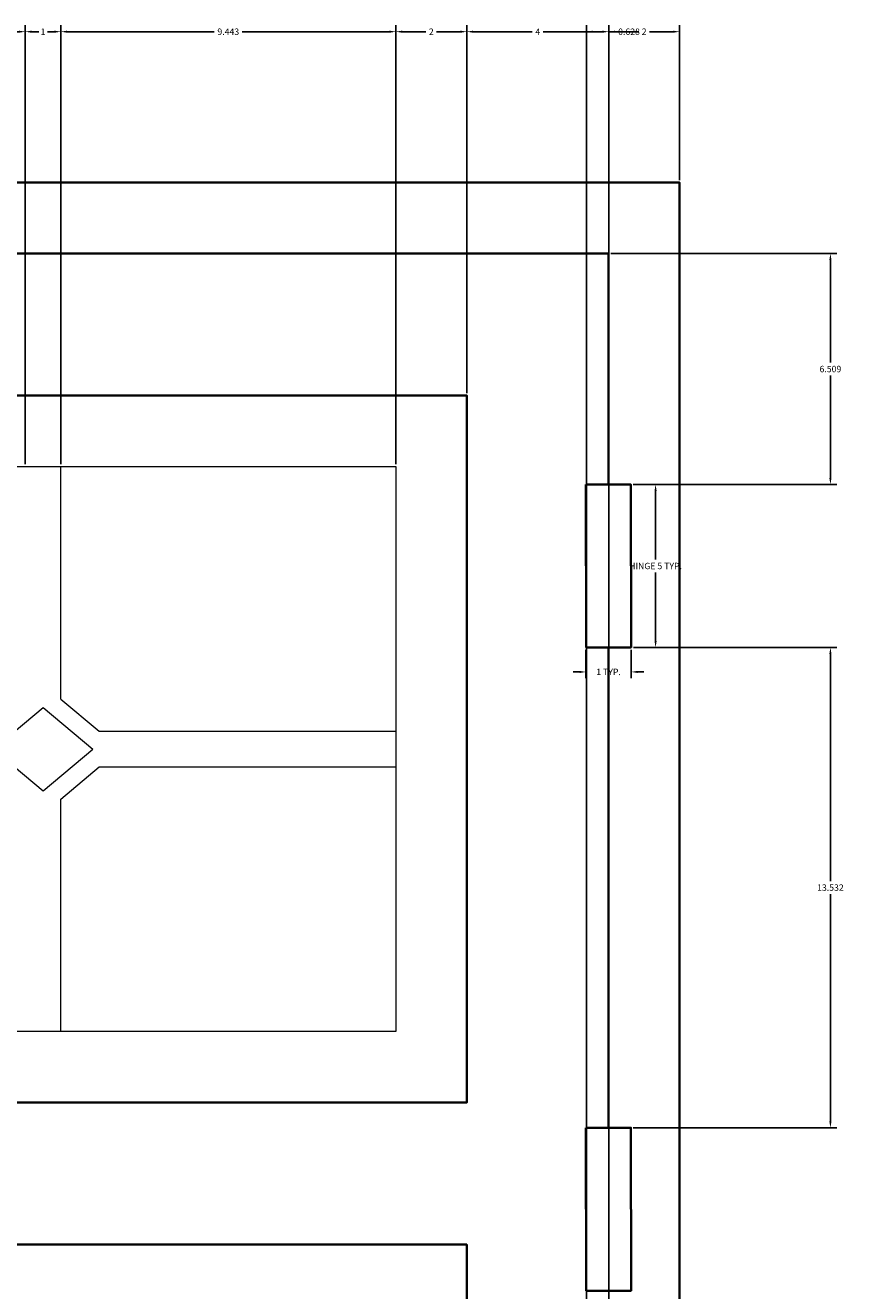
# Model space of a CAD drawing. Units: inches. Extents: x 3137 to 3299, y 1994 to 2089.
# Tile 7 of 14: x 3171 to 3194, y 2052 to 2087. Entities that reach past the tile are written whole.
import ezdxf

# ---------------------------------------------------------------- set-up
doc = ezdxf.new("R2010")
doc.units = ezdxf.units.IN
doc.header["$MEASUREMENT"] = 0
for name, color, linetype, lineweight in [('A-ANNO-DIMS', 2, 'Continuous', 18), ('A-DOOR', 4, 'Continuous', 35), ('A-GLAZ', 3, 'Continuous', 18)]:
    doc.layers.add(name, color=color, linetype=linetype, lineweight=lineweight)
doc.styles.get("Standard").update_dxf_attribs({"font": 'arial.ttf'})
doc.dimstyles.get("Standard").update_dxf_attribs({"dimtxt": 0.18, "dimasz": 0.18, "dimexe": 0.18, "dimexo": 0.0625, "dimgap": 0.09, "dimtad": 0, "dimtih": 1, "dimtoh": 1, "dimdec": 4, "dimzin": 0, "dimdsep": 46, "dimtxsty": 'Standard', "dimcen": 0.09, "dimadec": 0, "dimazin": 0, "dimtfac": 1, "dimtdec": 4, "dimtofl": 0, "dimtmove": 0, "dimatfit": 3, "dimfxl": 1, "dimtolj": 1, "dimtzin": 0, "dimarcsym": 0})

# ---------------------------------------------------------------- blocks, each defined once
blk = doc.blocks.new('GLAZ-DIAMOND-MOTIF')
for points in [[(0, 1.174), (1.407, 2.349)], [(1.407, 2.349), (2.809, 1.174)], [(0, 1.174), (1.407, 0)], [(1.407, 0), (2.809, 1.174)]]:
    blk.add_lwpolyline(points)
blk = doc.blocks.new('DOOR-HINGE')
blk.add_lwpolyline([(0, 4.592), (1.268, 4.592), (1.275, 0), (0.007, 0)], close=True)
blk = doc.blocks.new('*D5')
at = {"layer": 'A-ANNO-DIMS', "color": 0, "lineweight": -2, "transparency": 16777216}
for p, q in [((3188.174, 2074.365), (3188.98, 2074.365)), ((3188.8, 2074.185), (3188.8, 2072.252)), ((3188.8, 2069.953), (3188.8, 2071.886)), ((3188.174, 2069.773), (3188.98, 2069.773))]:
    blk.add_line(p, q, dxfattribs=at)
at = {"layer": 'A-ANNO-DIMS', "color": 0, "transparency": 16777216}
for points in [[(3188.77, 2074.185), (3188.83, 2074.185), (3188.8, 2074.365)], [(3188.77, 2069.953), (3188.83, 2069.953), (3188.8, 2069.773)]]:
    blk.add_solid(points, dxfattribs=at)
at = {"layer": 'Defpoints', "color": 0, "transparency": 16777216}
for p in [(3188.112, 2074.365), (3188.8, 2074.365), (3188.112, 2069.773)]:
    blk.add_point(p, dxfattribs=at)
at = {"layer": 'A-ANNO-DIMS', "color": 0, "transparency": 16777216, "insert": (3188.8, 2072.069), "char_height": 0.18, "attachment_point": 5}
blk.add_mtext('\\A1;HINGE 5 TYP.', dxfattribs=at)
blk = doc.blocks.new('*D6')
at = {"layer": 'A-ANNO-DIMS', "color": 0, "lineweight": -2, "transparency": 16777216}
for p, q in [((3186.837, 2069.711), (3186.837, 2068.904)), ((3188.112, 2069.711), (3188.112, 2068.904)), ((3186.657, 2069.084), (3186.477, 2069.084)), ((3188.292, 2069.084), (3188.472, 2069.084))]:
    blk.add_line(p, q, dxfattribs=at)
at = {"layer": 'A-ANNO-DIMS', "color": 0, "transparency": 16777216}
for points in [[(3186.657, 2069.114), (3186.657, 2069.054), (3186.837, 2069.084)], [(3188.292, 2069.114), (3188.292, 2069.054), (3188.112, 2069.084)]]:
    blk.add_solid(points, dxfattribs=at)
at = {"layer": 'Defpoints', "color": 0, "transparency": 16777216}
for p in [(3186.837, 2069.773), (3188.112, 2069.773), (3188.112, 2069.084)]:
    blk.add_point(p, dxfattribs=at)
at = {"layer": 'A-ANNO-DIMS', "color": 0, "transparency": 16777216, "insert": (3187.475, 2069.084), "char_height": 0.18, "attachment_point": 5}
blk.add_mtext('\\A1;1 TYP.', dxfattribs=at)
blk = doc.blocks.new('*D28')
at = {"layer": 'A-ANNO-DIMS', "color": 0, "lineweight": -2, "transparency": 16777216}
for p, q in [((3159.858, 2074.936), (3159.858, 2087.304)), ((3171.035, 2074.936), (3171.035, 2087.304)), ((3160.038, 2087.124), (3164.991, 2087.124)), ((3170.855, 2087.124), (3165.902, 2087.124))]:
    blk.add_line(p, q, dxfattribs=at)
at = {"layer": 'A-ANNO-DIMS', "color": 0, "transparency": 16777216}
for points in [[(3160.038, 2087.154), (3160.038, 2087.094), (3159.858, 2087.124)], [(3170.855, 2087.154), (3170.855, 2087.094), (3171.035, 2087.124)]]:
    blk.add_solid(points, dxfattribs=at)
at = {"layer": 'Defpoints', "color": 0, "transparency": 16777216}
for p in [(3171.035, 2087.124), (3159.858, 2074.874), (3171.035, 2074.874)]:
    blk.add_point(p, dxfattribs=at)
at = {"layer": 'A-ANNO-DIMS', "color": 0, "transparency": 16777216, "insert": (3165.446, 2087.124), "char_height": 0.18, "attachment_point": 5}
blk.add_mtext('\\A1;11.177', dxfattribs=at)
blk = doc.blocks.new('*D29')
at = {"layer": 'A-ANNO-DIMS', "color": 0, "lineweight": -2, "transparency": 16777216}
for p, q in [((3171.035, 2074.936), (3171.035, 2087.304)), ((3172.035, 2074.936), (3172.035, 2087.304)), ((3171.215, 2087.124), (3171.412, 2087.124)), ((3171.855, 2087.124), (3171.658, 2087.124))]:
    blk.add_line(p, q, dxfattribs=at)
at = {"layer": 'A-ANNO-DIMS', "color": 0, "transparency": 16777216}
for points in [[(3171.215, 2087.154), (3171.215, 2087.094), (3171.035, 2087.124)], [(3171.855, 2087.154), (3171.855, 2087.094), (3172.035, 2087.124)]]:
    blk.add_solid(points, dxfattribs=at)
at = {"layer": 'Defpoints', "color": 0, "transparency": 16777216}
for p in [(3172.035, 2087.124), (3171.035, 2074.874), (3172.035, 2074.874)]:
    blk.add_point(p, dxfattribs=at)
at = {"layer": 'A-ANNO-DIMS', "color": 0, "transparency": 16777216, "insert": (3171.535, 2087.124), "char_height": 0.18, "attachment_point": 5}
blk.add_mtext('\\A1;1', dxfattribs=at)
blk = doc.blocks.new('*D30')
at = {"layer": 'A-ANNO-DIMS', "color": 0, "lineweight": -2, "transparency": 16777216}
for p, q in [((3172.035, 2074.936), (3172.035, 2087.304)), ((3181.478, 2074.936), (3181.478, 2087.304)), ((3172.215, 2087.124), (3176.363, 2087.124)), ((3181.298, 2087.124), (3177.15, 2087.124))]:
    blk.add_line(p, q, dxfattribs=at)
at = {"layer": 'A-ANNO-DIMS', "color": 0, "transparency": 16777216}
for points in [[(3172.215, 2087.154), (3172.215, 2087.094), (3172.035, 2087.124)], [(3181.298, 2087.154), (3181.298, 2087.094), (3181.478, 2087.124)]]:
    blk.add_solid(points, dxfattribs=at)
at = {"layer": 'Defpoints', "color": 0, "transparency": 16777216}
for p in [(3181.478, 2087.124), (3172.035, 2074.874), (3181.478, 2074.874)]:
    blk.add_point(p, dxfattribs=at)
at = {"layer": 'A-ANNO-DIMS', "color": 0, "transparency": 16777216, "insert": (3176.756, 2087.124), "char_height": 0.18, "attachment_point": 5}
blk.add_mtext('\\A1;9.443', dxfattribs=at)
blk = doc.blocks.new('*D31')
at = {"layer": 'A-ANNO-DIMS', "color": 0, "lineweight": -2, "transparency": 16777216}
for p, q in [((3181.478, 2074.936), (3181.478, 2087.304)), ((3183.478, 2076.936), (3183.478, 2087.304)), ((3181.658, 2087.124), (3182.328, 2087.124)), ((3183.298, 2087.124), (3182.627, 2087.124))]:
    blk.add_line(p, q, dxfattribs=at)
at = {"layer": 'A-ANNO-DIMS', "color": 0, "transparency": 16777216}
for points in [[(3181.658, 2087.154), (3181.658, 2087.094), (3181.478, 2087.124)], [(3183.298, 2087.154), (3183.298, 2087.094), (3183.478, 2087.124)]]:
    blk.add_solid(points, dxfattribs=at)
at = {"layer": 'Defpoints', "color": 0, "transparency": 16777216}
for p in [(3183.478, 2087.124), (3183.478, 2076.874), (3181.478, 2074.874)]:
    blk.add_point(p, dxfattribs=at)
at = {"layer": 'A-ANNO-DIMS', "color": 0, "transparency": 16777216, "insert": (3182.478, 2087.124), "char_height": 0.18, "attachment_point": 5}
blk.add_mtext('\\A1;2', dxfattribs=at)
blk = doc.blocks.new('*D32')
at = {"layer": 'A-ANNO-DIMS', "color": 0, "lineweight": -2, "transparency": 16777216}
for p, q in [((3183.478, 2076.936), (3183.478, 2087.304)), ((3187.478, 2080.936), (3187.478, 2087.304)), ((3183.658, 2087.124), (3185.325, 2087.124)), ((3187.298, 2087.124), (3185.63, 2087.124))]:
    blk.add_line(p, q, dxfattribs=at)
at = {"layer": 'A-ANNO-DIMS', "color": 0, "transparency": 16777216}
for points in [[(3183.658, 2087.154), (3183.658, 2087.094), (3183.478, 2087.124)], [(3187.298, 2087.154), (3187.298, 2087.094), (3187.478, 2087.124)]]:
    blk.add_solid(points, dxfattribs=at)
at = {"layer": 'Defpoints', "color": 0, "transparency": 16777216}
for p in [(3187.478, 2087.124), (3187.478, 2080.874), (3183.478, 2076.874)]:
    blk.add_point(p, dxfattribs=at)
at = {"layer": 'A-ANNO-DIMS', "color": 0, "transparency": 16777216, "insert": (3185.478, 2087.124), "char_height": 0.18, "attachment_point": 5}
blk.add_mtext('\\A1;4', dxfattribs=at)
blk = doc.blocks.new('*D33')
at = {"layer": 'A-ANNO-DIMS', "color": 0, "lineweight": -2, "transparency": 16777216}
for p, q in [((3187.478, 2080.936), (3187.478, 2087.304)), ((3189.478, 2082.936), (3189.478, 2087.304)), ((3187.658, 2087.124), (3188.328, 2087.124)), ((3189.298, 2087.124), (3188.627, 2087.124))]:
    blk.add_line(p, q, dxfattribs=at)
at = {"layer": 'A-ANNO-DIMS', "color": 0, "transparency": 16777216}
for points in [[(3187.658, 2087.154), (3187.658, 2087.094), (3187.478, 2087.124)], [(3189.298, 2087.154), (3189.298, 2087.094), (3189.478, 2087.124)]]:
    blk.add_solid(points, dxfattribs=at)
at = {"layer": 'Defpoints', "color": 0, "transparency": 16777216}
for p in [(3189.478, 2087.124), (3189.478, 2082.874), (3187.478, 2080.874)]:
    blk.add_point(p, dxfattribs=at)
at = {"layer": 'A-ANNO-DIMS', "color": 0, "transparency": 16777216, "insert": (3188.478, 2087.124), "char_height": 0.18, "attachment_point": 5}
blk.add_mtext('\\A1;2', dxfattribs=at)
blk = doc.blocks.new('*D53')
at = {"layer": 'A-ANNO-DIMS', "color": 0, "lineweight": -2, "transparency": 16777216}
for p, q in [((3188.174, 2069.773), (3193.908, 2069.773)), ((3193.728, 2069.593), (3193.728, 2063.189)), ((3193.728, 2056.421), (3193.728, 2062.825)), ((3188.168, 2056.241), (3193.908, 2056.241))]:
    blk.add_line(p, q, dxfattribs=at)
at = {"layer": 'A-ANNO-DIMS', "color": 0, "transparency": 16777216}
for points in [[(3193.698, 2069.593), (3193.758, 2069.593), (3193.728, 2069.773)], [(3193.698, 2056.421), (3193.758, 2056.421), (3193.728, 2056.241)]]:
    blk.add_solid(points, dxfattribs=at)
at = {"layer": 'Defpoints', "color": 0, "transparency": 16777216}
for p in [(3188.112, 2069.773), (3193.728, 2069.773), (3188.105, 2056.241)]:
    blk.add_point(p, dxfattribs=at)
at = {"layer": 'A-ANNO-DIMS', "color": 0, "transparency": 16777216, "insert": (3193.728, 2063.007), "char_height": 0.18, "attachment_point": 5}
blk.add_mtext('\\A1;13.532', dxfattribs=at)
blk = doc.blocks.new('*D54')
at = {"layer": 'A-ANNO-DIMS', "color": 0, "lineweight": -2, "transparency": 16777216}
for p, q in [((3187.54, 2080.874), (3193.908, 2080.874)), ((3193.728, 2080.694), (3193.728, 2077.801)), ((3193.728, 2074.545), (3193.728, 2077.438)), ((3188.168, 2074.365), (3193.908, 2074.365))]:
    blk.add_line(p, q, dxfattribs=at)
at = {"layer": 'A-ANNO-DIMS', "color": 0, "transparency": 16777216}
for points in [[(3193.698, 2080.694), (3193.758, 2080.694), (3193.728, 2080.874)], [(3193.698, 2074.545), (3193.758, 2074.545), (3193.728, 2074.365)]]:
    blk.add_solid(points, dxfattribs=at)
at = {"layer": 'Defpoints', "color": 0, "transparency": 16777216}
for p in [(3187.478, 2080.874), (3193.728, 2080.874), (3188.105, 2074.365)]:
    blk.add_point(p, dxfattribs=at)
at = {"layer": 'A-ANNO-DIMS', "color": 0, "transparency": 16777216, "insert": (3193.728, 2077.619), "char_height": 0.18, "attachment_point": 5}
blk.add_mtext('\\A1;6.509', dxfattribs=at)
blk = doc.blocks.new('*D76')
at = {"layer": 'A-ANNO-DIMS', "color": 0, "lineweight": -2, "transparency": 16777216}
for p, q in [((3186.849, 2012.332), (3186.849, 2087.304)), ((3187.478, 2012.332), (3187.478, 2087.304)), ((3187.029, 2087.124), (3187.298, 2087.124)), ((3187.478, 2087.124), (3187.658, 2087.124))]:
    blk.add_line(p, q, dxfattribs=at)
at = {"layer": 'A-ANNO-DIMS', "color": 0, "transparency": 16777216}
for points in [[(3187.029, 2087.154), (3187.029, 2087.094), (3186.849, 2087.124)], [(3187.298, 2087.154), (3187.298, 2087.094), (3187.478, 2087.124)]]:
    blk.add_solid(points, dxfattribs=at)
at = {"layer": 'Defpoints', "color": 0, "transparency": 16777216}
for p in [(3187.478, 2087.124), (3186.849, 2012.269), (3187.478, 2012.269)]:
    blk.add_point(p, dxfattribs=at)
at = {"layer": 'A-ANNO-DIMS', "color": 0, "transparency": 16777216, "insert": (3188.052, 2087.124), "char_height": 0.18, "attachment_point": 5}
blk.add_mtext('\\A1;0.628', dxfattribs=at)

msp = doc.modelspace()

# ---------------------------------------------------------------- linework, layer by layer
at = {"layer": 'A-DOOR'}
for points in [[(3141.4777, 2082.874), (3189.4777, 2082.874), (3189.4777, 1998.874), (3141.4777, 1998.874)], [(3147.4777, 2056.9483), (3147.4777, 2076.874), (3183.4777, 2076.874), (3183.4777, 2056.9483)], [(3147.4777, 2032.1375), (3147.4777, 2052.9483), (3183.4777, 2052.9483), (3183.4777, 2032.1375)]]:
    msp.add_lwpolyline(points, close=True, dxfattribs=at)
for points in [[(3187.4777, 2007.6773), (3187.4777, 2000.874), (3143.4777, 2000.874), (3143.4777, 2080.874), (3187.4777, 2080.874), (3187.4777, 2076.298)], [(3187.4777, 2080.874), (3187.4777, 2074.365)], [(3187.4777, 2069.7731), (3187.4777, 2056.2413)], [(3187.3375, 2056.2413), (3187.6053, 2056.2413)]]:
    msp.add_lwpolyline(points, dxfattribs=at)
at = {"layer": 'A-GLAZ'}
for p, q in [((3172.0351, 2068.3193), (3172.0351, 2074.874)), ((3173.1196, 2067.4111), (3181.4777, 2067.4111)), ((3173.1196, 2066.4111), (3181.4777, 2066.4111)), ((3172.0351, 2058.9483), (3172.0351, 2065.5029))]:
    msp.add_line(p, q, dxfattribs=at)
msp.add_lwpolyline([(3149.4777, 2058.9483), (3149.4777, 2074.874), (3181.4777, 2074.874), (3181.4777, 2058.9483)], close=True, dxfattribs=at)
for points in [[(3172.0351, 2068.3193), (3173.1196, 2067.4111)], [(3172.0351, 2065.5029), (3173.1196, 2066.4111)]]:
    msp.add_lwpolyline(points, dxfattribs=at)

# ---------------------------------------------------------------- block references
at = {"layer": 'A-DOOR'}
for p in [(3186.837, 2069.773), (3186.837, 2051.6493)]:
    msp.add_blockref('DOOR-HINGE', p, dxfattribs=at)
at = {"layer": 'A-GLAZ'}
msp.add_blockref('GLAZ-DIAMOND-MOTIF', (3170.1284, 2065.737), dxfattribs=at)

# ---------------------------------------------------------------- dimensions: what is measured, and where the dimension line sits
at = {"layer": 'A-ANNO-DIMS'}
for base, p1, p2, override, picture, middle in [((3171.0351, 2087.124), (3159.8577, 2074.874), (3171.0351, 2074.874), {"dimdec": 3, "dimlfac": 1, "dimrnd": 0, "dimzin": 0, "dimdsep": 46, "dimlunit": 2}, '*D28', (3165.4464, 2087.124)), ((3172.0351, 2087.124), (3171.0351, 2074.874), (3172.0351, 2074.874), {"dimdec": 0, "dimlfac": 1, "dimrnd": 0, "dimzin": 0, "dimdsep": 46, "dimlunit": 2}, '*D29', (3171.5351, 2087.124)), ((3181.4777, 2087.124), (3172.0351, 2074.874), (3181.4777, 2074.874), {"dimdec": 3, "dimlfac": 1, "dimrnd": 0, "dimzin": 0, "dimdsep": 46, "dimlunit": 2}, '*D30', (3176.7564, 2087.124)), ((3183.4777, 2087.124), (3181.4777, 2074.874), (3183.4777, 2076.874), {"dimdec": 0, "dimlfac": 1, "dimrnd": 0, "dimzin": 0, "dimdsep": 46, "dimlunit": 2}, '*D31', (3182.4777, 2087.124)), ((3187.4777, 2087.124), (3183.4777, 2076.874), (3187.4777, 2080.874), {"dimdec": 0, "dimlfac": 1, "dimrnd": 0, "dimzin": 0, "dimdsep": 46, "dimlunit": 2}, '*D32', (3185.4777, 2087.124)), ((3187.4777, 2087.124), (3186.8495, 2012.2692), (3187.4777, 2012.2692), {"dimdec": 3, "dimlfac": 1, "dimrnd": 0, "dimzin": 0, "dimdsep": 46, "dimlunit": 2}, '*D76', (3188.0516, 2087.124)), ((3189.4777, 2087.124), (3187.4777, 2080.874), (3189.4777, 2082.874), {"dimdec": 0, "dimlfac": 1, "dimrnd": 0, "dimzin": 0, "dimdsep": 46, "dimlunit": 2}, '*D33', (3188.4777, 2087.124))]:
    dim = msp.add_linear_dim(base=base, p1=p1, p2=p2, dimstyle='Standard', override=override, dxfattribs=at)
    dim.commit()
    dim.dimension.update_dxf_attribs({"geometry": picture, "text_midpoint": middle})
for base, p1, p2, picture, middle in [((3193.7277, 2080.874), (3188.1053, 2074.365), (3187.4777, 2080.874), '*D54', (3193.7277, 2077.6195)), ((3193.7277, 2069.7731), (3188.1053, 2056.2413), (3188.1116, 2069.7731), '*D53', (3193.7277, 2063.0072))]:
    dim = msp.add_linear_dim(base=base, p1=p1, p2=p2, angle=90, dimstyle='Standard', override={"dimdec": 3, "dimlfac": 1, "dimrnd": 0, "dimzin": 0, "dimdsep": 46, "dimlunit": 2}, dxfattribs=at)
    dim.commit()
    dim.dimension.update_dxf_attribs({"geometry": picture, "text_midpoint": middle})
dim = msp.add_linear_dim(base=(3188.8004, 2074.365), p1=(3188.1116, 2069.7731), p2=(3188.1116, 2074.365), angle=90, text='HINGE <> TYP.', dimstyle='Standard', override={"dimdec": 0, "dimrnd": 0, "dimzin": 0, "dimlunit": 2}, dxfattribs=at)
dim.commit()
dim.dimension.update_dxf_attribs({"geometry": '*D5', "text_midpoint": (3188.8004, 2072.0691)})
dim = msp.add_linear_dim(base=(3188.1116, 2069.0843), p1=(3186.8375, 2069.7731), p2=(3188.1116, 2069.7731), text='<> TYP.', dimstyle='Standard', override={"dimdec": 0, "dimrnd": 0, "dimzin": 0, "dimlunit": 2}, dxfattribs=at)
dim.commit()
dim.dimension.update_dxf_attribs({"geometry": '*D6', "text_midpoint": (3187.4745, 2069.0843)})

doc.saveas('drawing.dxf')
